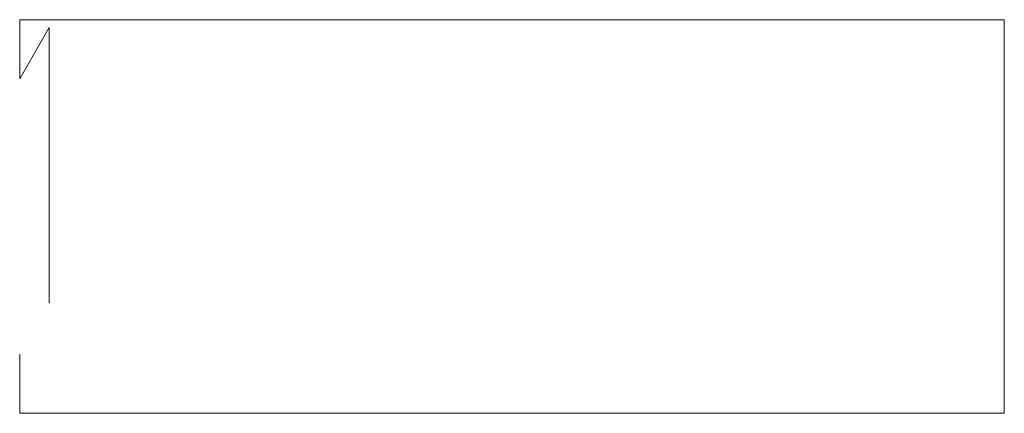
# Model space of a CAD drawing. Units: millimetres. Extents: x -288 to 383, y -34 to 128.
# Tile 1 of 1: x 182.5 to 382.5, y 48.2 to 128.2. Entities that reach past the tile are written whole.
import ezdxf

# ---------------------------------------------------------------- set-up
doc = ezdxf.new("R2010")
doc.units = ezdxf.units.MM
doc.layers.add('M-CONS', color=8, linetype='Continuous', lineweight=13)

msp = doc.modelspace()

# ---------------------------------------------------------------- linework, layer by layer
at = {"layer": 'M-CONS'}
for p, q in [((182.53, 128.19), (382.53, 128.19)), ((182.53, 128.19), (182.53, 116.19)), ((382.53, 128.19), (382.53, 48.19)), ((182.53, 116.19), (188.53, 126.58)), ((188.53, 126.58), (188.53, 70.58)), ((182.53, 48.19), (182.53, 60.19)), ((382.53, 48.19), (182.53, 48.19))]:
    msp.add_line(p, q, dxfattribs=at)

doc.saveas('drawing.dxf')
